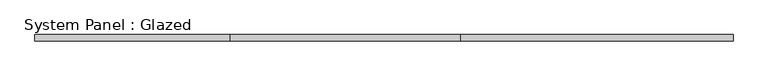
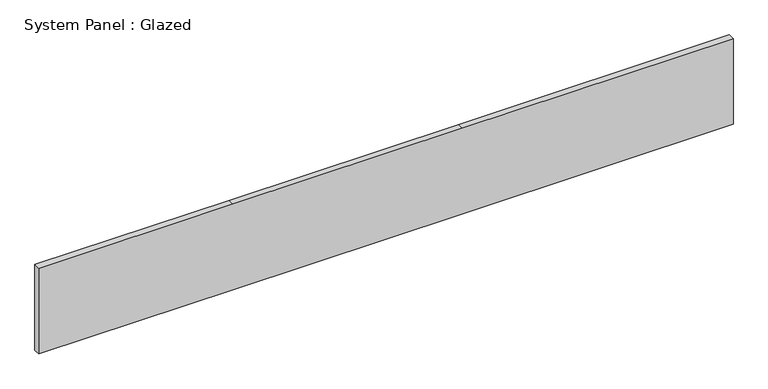
"""IFC4 building model written with IfcOpenShell, lengths in millimetres: plate geometry, System Panel : Glazed."""

from ifc_helpers import new_model, si_unit, frame, origin, place, context, project, spatial, polyline, outline, extrude, source, transform, mapped, element, save


def system_panel_glazed_c1b5d4b5(model_context):
    return source(origin(), model_context, "Body", "SweptSolid", [
        extrude(outline(polyline([(0.0, -1384.3), (0.0, -609.6), (0.0, 304.8), (0.0, 1384.3), (361.95, 1384.3), (361.95, 304.8), (361.95, -609.6), (361.95, -1384.3), (0.0, -1384.3)])), frame((0.0, 19.05, 0.0), z_axis=(0.0, 1.0, 0.0), x_axis=(0.0, 0.0, 1.0)), (0.0, 0.0, 1.0), 25.4),
    ])


if __name__ == "__main__":
    model = new_model("IFC4")
    model_context = context("Model", 3, world=origin())
    ifc_project = project(units=[si_unit("LENGTHUNIT", "METRE", prefix="MILLI")], contexts=[model_context])
    site = spatial("IfcSite", under=ifc_project)
    building = spatial("IfcBuilding", under=site)
    placement = place(None, origin())
    system_panel_glazed_shape = system_panel_glazed_c1b5d4b5(model_context)
    element("IfcPlate", 1, ObjectType="System Panel : Glazed", at=placement, inside=building, context=model_context, shape_type="MappedRepresentation", body=[
        mapped(system_panel_glazed_shape, transform((0.0, 0.0, 0.0), x_axis=(1.0, 0.0, 0.0), y_axis=(0.0, 1.0, 0.0), z_axis=(0.0, 0.0, 1.0))),
    ])
    save(model, "model.ifc")

# Revit data of these elements
# Type "System Panel : Glazed"
#   Construction Type Id = "GSP4R"
#   Analytic Construction = "1/8 in Pilkington single glazing"
#   Visual Light Transmittance = 0.9
#   Solar Heat Gain Coefficient = 0.86
#   Heat Transfer Coefficient (U) = 1.18115 BTU/(h·ft²·°F)
#   Define Thermal Properties by = 1
# Element 1 (IfcPlate, "System Panel : Glazed")
#   Materials on its faces: "Glass"
# Materials
#   "Glass": class "Glass", colour RGB 0 128 192, transparency 0.75, Description = "Soda Lime Glass", Cost = 0
